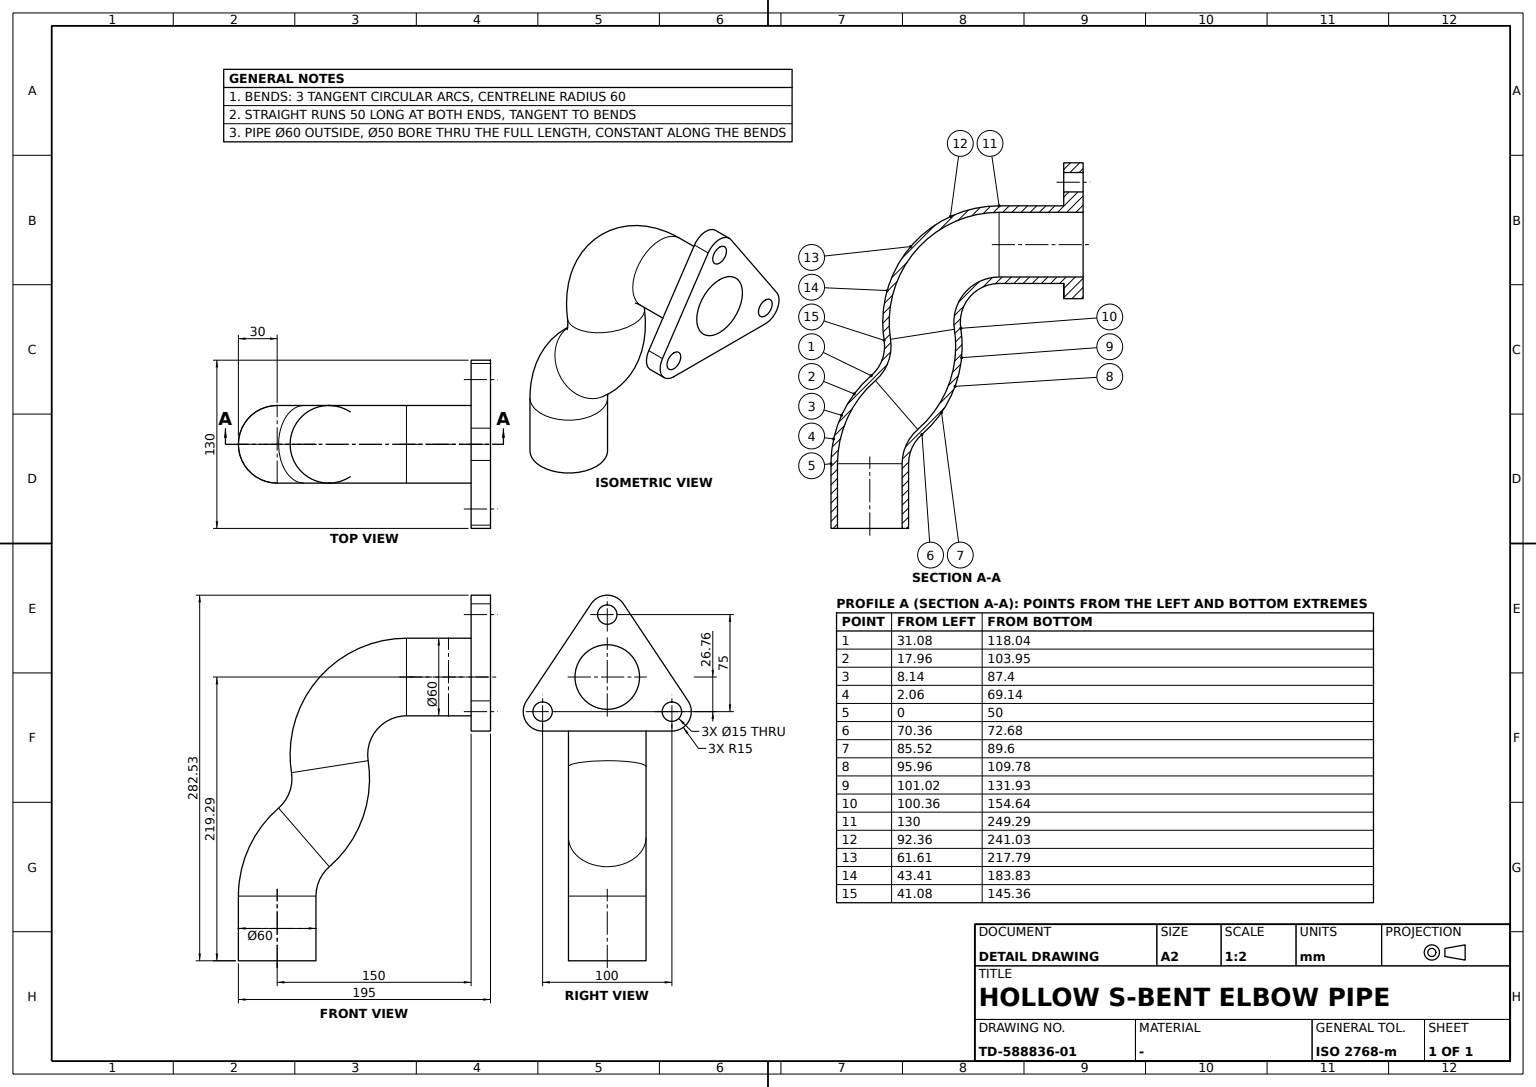
CATIA V5 part; units mm, degrees
sketch "Sketch2" plane through (0, 0, 0) normal (0, 0, 1) x (1, 0, 0)
  circle A0 centre (0, 0) radius 30
  dimension "radius A0" = 30
sketch "Sketch1" plane through (0, 0, 0) normal (1, 0, 0) x (0, 1, 0)
  line L0 (0, 0) -> (0, 50)
  arc A0 (0, 50) -> (20.7228, 95.3575) centre (60, 50) cw
  arc A1 (20.7228, 95.3575) -> (40.7228, 150) centre (-18.5544, 140.715) ccw
  point P0 (40.7228, 150)
  point P1 (150, 219.285)
  line L1 (150, 219.285) -> (100, 219.285)
  arc A2 (100, 219.285) -> (40.7228, 150) centre (100, 159.285) ccw
  dimension "length L0" = 50
  dimension "radius A0" = 60
  dimension "radius A1" = 60
  dimension "distance origin P0 y axis" = 150
  dimension "radius A2" = 60
  dimension "distance L0 P1" = 150
  dimension "length L1" = 50
  constraint vertical L0 y-axis
  constraint tangency A0 L0
  constraint tangency A1 A0
  constraint tangency A2 L1
  constraint tangency A1 A2
  constraint horizontal L1 x-axis
sweep "Rib1" add profiles "Sketch2" path "Sketch1"
sketch "Sketch3" plane through (0, 150, 0) normal (0, 1, 0) x (-1, 0, 0)
  line L0 (0, 0) -> (0, 298.728) construction
  line L1 (-50, 177.5259) -> (50, 177.5259)
  arc A0 (50, 177.5259) -> (62.4808, 200.8464) centre (50, 192.5259) ccw
  point P0 (50, 192.5259)
  line L2 (62.4808, 200.8464) -> (12.4808, 275.8464)
  arc A1 (12.4808, 275.8464) -> (-12.4808, 275.8464) centre (0, 267.5259) ccw
  point P1 (0, 267.5259)
  line L3 (-12.4808, 275.8464) -> (-62.4808, 200.8464)
  arc A2 (-62.4808, 200.8464) -> (-50, 177.5259) centre (-50, 192.5259) ccw
  point P2 (-50, 192.5259)
  circle A3 centre (0, 219.285) radius 41.7592 construction
  point P3 (0, 219.285)
  circle A4 centre (0, 219.285) radius 30 construction
  circle A5 centre (50, 192.5259) radius 7.5
  point P4 (50, 192.5259)
  circle A6 centre (-50, 192.5259) radius 7.5
  circle A7 centre (0, 267.5259) radius 7.5
  point P5 (3.5077, 260.8967)
  dimension "radius A1" = 15
  dimension "radius A0" = 15
  dimension "radius A2" = 15
  dimension "distance P0 P1 y axis" = 75
  dimension "distance P1 P2 x axis" = 50
  dimension "radius A5" = 7.5
  dimension "radius A6" = 7.5
  dimension "radius A7" = 7.5
  constraint vertical L0 y-axis
  constraint horizontal L1 x-axis
  constraint tangency A0 L1
  constraint tangency A1 L2
  constraint tangency A2 L3
  constraint tangency L2 A0
  constraint tangency A1 L3
  constraint tangency A2 L1
  constraint tangency A3 L3
  constraint tangency A3 L2
  constraint tangency A3 L1
  constraint symmetry L3 L2 L0
  constraint coincidence P1 L0
  constraint coincidence A7 P5
  constraint coincidence P5 A3
  constraint coincidence P4 P0
  constraint concentricity P3 A4
extrude "Pad1" add sketch "Sketch3" along normal blind 15
sketch "Sketch4" plane through (0, 0, 0) normal (0, 0, -1) x (1, 0, 0)
  circle A0 centre (0, 0) radius 25
  dimension "radius A0" = 25
sweep "Slot1" cut profiles "Sketch4" path "Sketch1"
sketch "Sketch5" plane through (0, 165, 0) normal (0, 1, 0) x (-1, 0, 0)
  line L0 (0, 0) -> (0, 283.8811) construction
  circle A0 centre (0, 219.285) radius 25
  point P0 (0, 219.285)
  dimension "radius A0" = 25
  dimension "distance origin P0" = 219.285
  constraint vertical L0 y-axis
  constraint coincidence P0 L0
extrude "Pocket1" cut sketch "Sketch5" against normal blind 15
